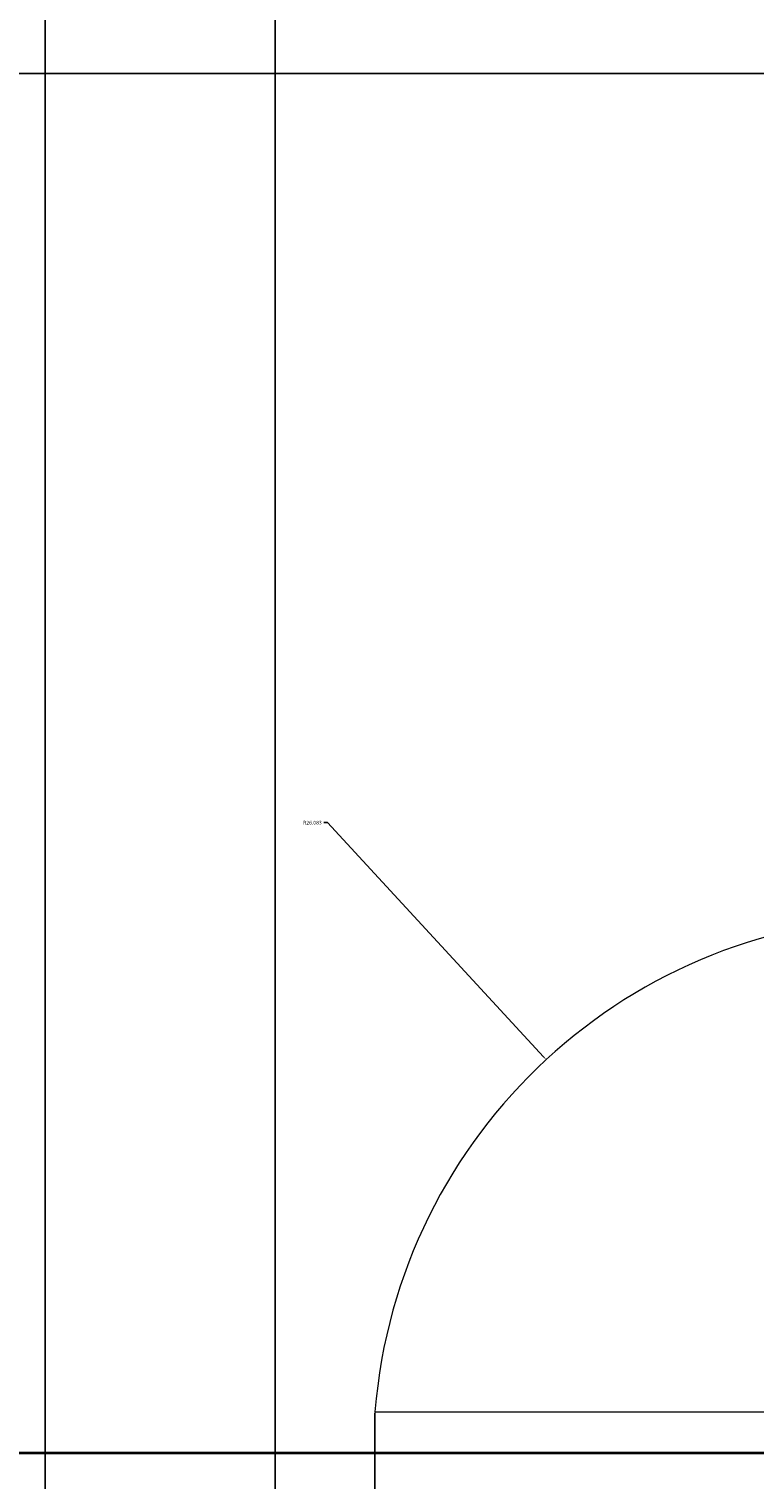
# Model space of a CAD drawing. Units: feet. Extents: x 1654 to 2985, y 1348 to 2230.
# Tile 9 of 53: x 1956 to 1991, y 1573 to 1643. Entities that reach past the tile are written whole.
import ezdxf

# ---------------------------------------------------------------- set-up
doc = ezdxf.new("R2010")
doc.units = ezdxf.units.FT
for name, color, linetype, lineweight in [('A-ANNO-DIMS', 2, 'Continuous', 18), ('A-DOOR', 3, 'Continuous', 18), ('A-WALL', 7, 'Continuous', 35)]:
    doc.layers.add(name, color=color, linetype=linetype, lineweight=lineweight)
doc.styles.get("Standard").update_dxf_attribs({"font": 'arial.ttf'})
doc.dimstyles.get("Standard").update_dxf_attribs({"dimtxt": 0.18, "dimasz": 0.18, "dimexe": 0.18, "dimexo": 0.0625, "dimgap": 0.09, "dimtad": 0, "dimtih": 1, "dimtoh": 1, "dimdec": 4, "dimzin": 0, "dimdsep": 46, "dimtxsty": 'Standard', "dimcen": 0.09, "dimadec": 0, "dimazin": 0, "dimtfac": 1, "dimtdec": 4, "dimtofl": 0, "dimtmove": 0, "dimatfit": 3, "dimfxl": 1, "dimtolj": 1, "dimtzin": 0, "dimarcsym": 0})

# ---------------------------------------------------------------- blocks, each defined once
blk = doc.blocks.new('DOOR-GUEST-ENTRY')
for p, q in [((-2, 26.083), (9, 26.083)), ((-26, 2.083), (9, 2.083))]:
    blk.add_line(p, q)
blk.add_arc((0, 0), 26.083, 90, 175.41878)
blk = doc.blocks.new('*D30')
at = {"layer": 'A-ANNO-DIMS', "color": 0, "lineweight": -2, "transparency": 16777216}
for p, q in [((1973.092, 1576.192), (1973.092, 1570.825)), ((2008.092, 1576.192), (2008.092, 1570.825)), ((1973.272, 1571.005), (1989.137, 1571.005)), ((2007.912, 1571.005), (1992.048, 1571.005))]:
    blk.add_line(p, q, dxfattribs=at)
at = {"layer": 'A-ANNO-DIMS', "color": 0, "transparency": 16777216}
for points in [[(1973.272, 1571.035), (1973.272, 1570.975), (1973.092, 1571.005)], [(2007.912, 1571.035), (2007.912, 1570.975), (2008.092, 1571.005)]]:
    blk.add_solid(points, dxfattribs=at)
at = {"layer": 'Defpoints', "color": 0, "transparency": 16777216}
for p in [(1973.092, 1576.255), (2008.092, 1576.255), (2008.092, 1571.005)]:
    blk.add_point(p, dxfattribs=at)
at = {"layer": 'A-ANNO-DIMS', "color": 0, "transparency": 16777216, "insert": (1990.592, 1571.005), "char_height": 0.18, "attachment_point": 5}
blk.add_mtext('\\A1;GUEST ENTRY 35 TYP.', dxfattribs=at)
blk = doc.blocks.new('*D90')
at = {"layer": 'A-ANNO-DIMS', "color": 0, "lineweight": -2, "transparency": 16777216}
for p, q in [((1852.155, 1641.187), (2242.272, 1641.187)), ((2242.092, 1641.007), (2242.092, 1607.903)), ((2242.092, 1574.435), (2242.092, 1607.539)), ((1852.155, 1574.255), (2242.272, 1574.255))]:
    blk.add_line(p, q, dxfattribs=at)
at = {"layer": 'A-ANNO-DIMS', "color": 0, "transparency": 16777216}
for points in [[(2242.062, 1641.007), (2242.122, 1641.007), (2242.092, 1641.187)], [(2242.062, 1574.435), (2242.122, 1574.435), (2242.092, 1574.255)]]:
    blk.add_solid(points, dxfattribs=at)
at = {"layer": 'Defpoints', "color": 0, "transparency": 16777216}
for p in [(1852.092, 1641.187), (2242.092, 1641.187), (1852.092, 1574.255)]:
    blk.add_point(p, dxfattribs=at)
at = {"layer": 'A-ANNO-DIMS', "color": 0, "transparency": 16777216, "insert": (2242.092, 1607.721), "char_height": 0.18, "attachment_point": 5}
blk.add_mtext('\\A1;66.93', dxfattribs=at)
blk = doc.blocks.new('*D97')
at = {"layer": 'A-ANNO-DIMS', "color": 0, "lineweight": -2, "transparency": 16777216}
for p, q in [((1957.092, 2108.192), (1957.092, 1534.075)), ((1968.254, 2108.192), (1968.254, 1534.075)), ((1957.272, 1534.255), (1962.219, 1534.255)), ((1968.074, 1534.255), (1963.128, 1534.255))]:
    blk.add_line(p, q, dxfattribs=at)
at = {"layer": 'A-ANNO-DIMS', "color": 0, "transparency": 16777216}
for points in [[(1957.272, 1534.285), (1957.272, 1534.225), (1957.092, 1534.255)], [(1968.074, 1534.285), (1968.074, 1534.225), (1968.254, 1534.255)]]:
    blk.add_solid(points, dxfattribs=at)
at = {"layer": 'Defpoints', "color": 0, "transparency": 16777216}
for p in [(1957.092, 2108.255), (1968.254, 2108.255), (1968.254, 1534.255)]:
    blk.add_point(p, dxfattribs=at)
at = {"layer": 'A-ANNO-DIMS', "color": 0, "transparency": 16777216, "insert": (1962.673, 1534.255), "char_height": 0.18, "attachment_point": 5}
blk.add_mtext('\\A1;11.162', dxfattribs=at)
blk = doc.blocks.new('*D105')
at = {"layer": 'A-ANNO-DIMS', "color": 0, "lineweight": -2, "transparency": 16777216}
for p, q in [((1970.606, 1604.838), (1970.786, 1604.838)), ((1970.786, 1604.838), (1981.279, 1593.47)), ((1999.002, 1574.172), (1999.182, 1574.172)), ((1999.092, 1574.082), (1999.092, 1574.262))]:
    blk.add_line(p, q, dxfattribs=at)
at = {"layer": 'A-ANNO-DIMS', "color": 0, "transparency": 16777216}
blk.add_solid([(1981.301, 1593.491), (1981.257, 1593.45), (1981.401, 1593.338)], dxfattribs=at)
at = {"layer": 'Defpoints', "color": 0, "transparency": 16777216}
for p in [(1981.401, 1593.338), (1999.092, 1574.172)]:
    blk.add_point(p, dxfattribs=at)
at = {"layer": 'A-ANNO-DIMS', "color": 0, "transparency": 16777216, "insert": (1970.056, 1604.838), "char_height": 0.18, "attachment_point": 5}
blk.add_mtext('\\A1;R26.083', dxfattribs=at)

msp = doc.modelspace()

# ---------------------------------------------------------------- linework, layer by layer
at = {"layer": 'A-WALL'}
msp.add_line((1852.0924, 1574.2549), (1999.0924, 1574.2549), dxfattribs=at)

# ---------------------------------------------------------------- block references
at = {"layer": 'A-DOOR'}
msp.add_blockref('DOOR-GUEST-ENTRY', (1999.0924, 1574.1716), dxfattribs=at)

# ---------------------------------------------------------------- dimensions: what is measured, and where the dimension line sits
at = {"layer": 'A-ANNO-DIMS'}
dim = msp.add_linear_dim(base=(1968.2542, 1534.2549), p1=(1957.0924, 2108.2549), p2=(1968.2542, 2108.2549), dimstyle='Standard', override={"dimdec": 3, "dimlfac": 1, "dimrnd": 0, "dimzin": 0, "dimdsep": 46, "dimlunit": 2}, dxfattribs=at)
dim.commit()
dim.dimension.update_dxf_attribs({"geometry": '*D97', "text_midpoint": (1962.6733, 1534.2549)})
dim = msp.add_linear_dim(base=(2242.0924, 1641.187), p1=(1852.0924, 1574.2549), p2=(1852.0924, 1641.187), angle=90, dimstyle='Standard', override={"dimdec": 2, "dimlfac": 1, "dimrnd": 0, "dimzin": 0, "dimdsep": 46, "dimlunit": 2}, dxfattribs=at)
dim.commit()
dim.dimension.update_dxf_attribs({"geometry": '*D90', "text_midpoint": (2242.0924, 1607.721)})
dim = msp.add_radius_dim(center=(1999.0924, 1574.1716), mpoint=(1981.401, 1593.338), dimstyle='Standard', override={"dimdec": 3, "dimlfac": 1, "dimrnd": 0, "dimzin": 0, "dimdsep": 46, "dimlunit": 2}, dxfattribs=at)
dim.commit()
dim.dimension.update_dxf_attribs({"geometry": '*D105', "text_midpoint": (1970.0563, 1604.8379), "dimtype": 164})
dim = msp.add_linear_dim(base=(2008.0924, 1571.0049), p1=(1973.0924, 1576.2549), p2=(2008.0924, 1576.2549), text='GUEST ENTRY <> TYP.', dimstyle='Standard', override={"dimdec": 0, "dimlfac": 1, "dimrnd": 0, "dimzin": 0, "dimdsep": 46, "dimlunit": 2}, dxfattribs=at)
dim.commit()
dim.dimension.update_dxf_attribs({"geometry": '*D30', "text_midpoint": (1990.5924, 1571.0049)})

doc.saveas('drawing.dxf')
